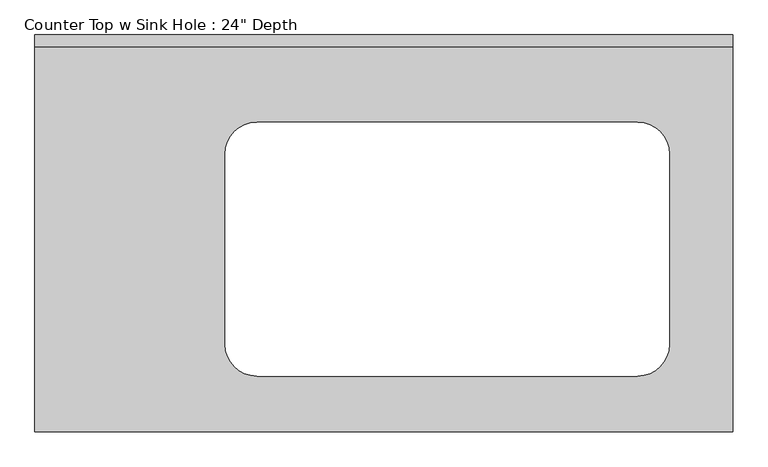
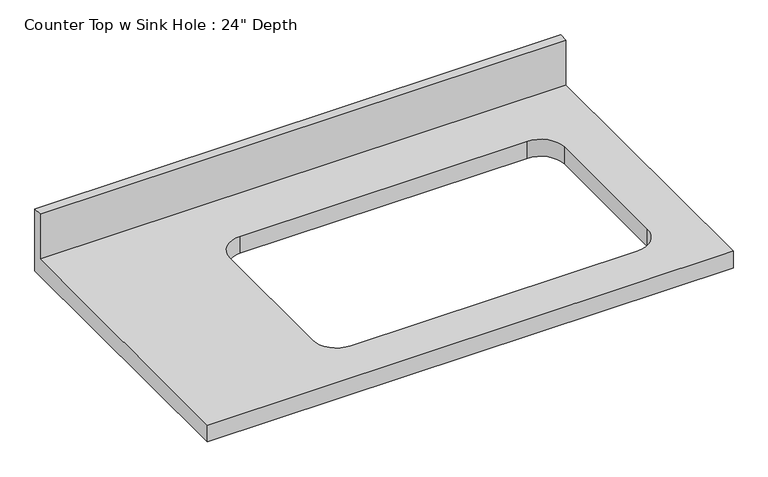
"""IFC4 building model written with IfcOpenShell, lengths in millimetres: furniture geometry."""

from ifc_helpers import new_model, si_unit, frame, origin, place, context, project, spatial, polyline, circle_curve, source, transform, mapped, element, save
from ifc_brep_helpers import plane_surface, revolved_surface, advanced_brep


def furniture_a6d59748(model_context):
    return source(origin(), model_context, "Body", "AdvancedBrep", [
        advanced_brep(
        [(-1200.4622951, -635.0, 914.4), (-82.8622951, -635.0, 914.4), (-82.8622951, -19.05, 914.4), (-1200.4622951, -19.05, 914.4), (-844.8622951, -139.7, 914.4), (-235.2622951, -139.7, 914.4), (-184.4622951, -190.5, 914.4), (-184.4622951, -495.3, 914.4), (-235.2622951, -546.1, 914.4), (-844.8622951, -546.1, 914.4), (-895.6622951, -495.3, 914.4), (-895.6622951, -190.5, 914.4), (-82.8622951, 0.0, 876.3), (-82.8622951, -635.0, 876.3), (-1200.4622951, -635.0, 876.3), (-1200.4622951, 0.0, 876.3), (-235.2622951, -139.7, 876.3), (-844.8622951, -139.7, 876.3), (-895.6622951, -190.5, 876.3), (-895.6622951, -495.3, 876.3), (-844.8622951, -546.1, 876.3), (-235.2622951, -546.1, 876.3), (-184.4622951, -495.3, 876.3), (-184.4622951, -190.5, 876.3), (-1200.4622951, 0.0, 1016.0), (-82.8622951, 0.0, 1016.0), (-1200.4622951, -19.05, 1016.0), (-82.8622951, -19.05, 1016.0)],
        [
            (0, 1),
            (1, 2),
            (2, 3),
            (3, 0),
            (4, 5),
            (5, 6, circle_curve(frame((-235.2622951, -190.5, 914.4), z_axis=(0.0, 0.0, -1.0), x_axis=(1.0, 0.0, 0.0)), 50.8)),
            (6, 7),
            (7, 8, circle_curve(frame((-235.2622951, -495.3, 914.4), z_axis=(0.0, 0.0, -1.0), x_axis=(1.0, 0.0, 0.0)), 50.8)),
            (8, 9),
            (9, 10, circle_curve(frame((-844.8622951, -495.3, 914.4), z_axis=(0.0, 0.0, -1.0), x_axis=(1.0, 0.0, 0.0)), 50.8)),
            (10, 11),
            (11, 4, circle_curve(frame((-844.8622951, -190.5, 914.4), z_axis=(0.0, 0.0, -1.0), x_axis=(1.0, 0.0, 0.0)), 50.8)),
            (12, 13),
            (13, 14),
            (14, 15),
            (15, 12),
            (16, 17),
            (17, 18, circle_curve(frame((-844.8622951, -190.5, 876.3), z_axis=(0.0, 0.0, 1.0), x_axis=(1.0, 0.0, 0.0)), 50.8)),
            (18, 19),
            (19, 20, circle_curve(frame((-844.8622951, -495.3, 876.3), z_axis=(0.0, 0.0, 1.0), x_axis=(1.0, 0.0, 0.0)), 50.8)),
            (20, 21),
            (21, 22, circle_curve(frame((-235.2622951, -495.3, 876.3), z_axis=(0.0, 0.0, 1.0), x_axis=(1.0, 0.0, 0.0)), 50.8)),
            (22, 23),
            (23, 16, circle_curve(frame((-235.2622951, -190.5, 876.3), z_axis=(0.0, 0.0, 1.0), x_axis=(1.0, 0.0, 0.0)), 50.8)),
            (15, 24),
            (24, 25),
            (25, 12),
            (14, 0),
            (3, 26),
            (26, 24),
            (13, 1),
            (25, 27),
            (27, 2),
            (26, 27),
            (4, 17),
            (16, 5),
            (11, 18),
            (10, 19),
            (9, 20),
            (8, 21),
            (7, 22),
            (6, 23),
        ],
        [
            plane_surface(frame((-1200.4622951, 0.0, 914.4), z_axis=(0.0, 0.0, 1.0), x_axis=(-1.0, 0.0, 0.0))),
            plane_surface(frame((-1200.4622951, 0.0, 876.3), z_axis=(0.0, 0.0, -1.0), x_axis=(1.0, 0.0, 0.0))),
            plane_surface(frame((-82.8622951, 0.0, 914.4), z_axis=(0.0, 1.0, 0.0), x_axis=(0.0, 0.0, -1.0))),
            plane_surface(frame((-1200.4622951, 0.0, 914.4), z_axis=(-1.0, 0.0, 0.0), x_axis=(0.0, 0.0, -1.0))),
            plane_surface(frame((-1200.4622951, -635.0, 914.4), z_axis=(0.0, -1.0, 0.0), x_axis=(0.0, 0.0, -1.0))),
            plane_surface(frame((-82.8622951, -635.0, 914.4), z_axis=(1.0, 0.0, 0.0), x_axis=(0.0, 0.0, -1.0))),
            plane_surface(frame((-1200.4622951, 0.0, 1016.0), z_axis=(0.0, 0.0, 1.0), x_axis=(0.0, -1.0, 0.0))),
            plane_surface(frame((-1200.4622951, -19.05, 1016.0), z_axis=(0.0, -1.0, 0.0), x_axis=(0.0, 0.0, -1.0))),
            plane_surface(frame((-235.2622951, -139.7, 914.4), z_axis=(0.0, -1.0, 0.0), x_axis=(0.0, 0.0, -1.0))),
            revolved_surface(polyline([(-794.0622951, -190.5, 914.4), (-794.0622951, -190.5, 876.3)]), (-844.8622951, -190.5, 876.3), (0.0, 0.0, 1.0)),
            plane_surface(frame((-895.6622951, -190.5, 914.4), z_axis=(1.0, 0.0, 0.0), x_axis=(0.0, 0.0, -1.0))),
            revolved_surface(polyline([(-794.0622951, -495.3, 914.4), (-794.0622951, -495.3, 876.3)]), (-844.8622951, -495.3, 876.3), (0.0, 0.0, 1.0)),
            plane_surface(frame((-844.8622951, -546.1, 914.4), z_axis=(0.0, 1.0, 0.0), x_axis=(0.0, 0.0, -1.0))),
            revolved_surface(polyline([(-184.4622951, -495.3, 914.4), (-184.4622951, -495.3, 876.3)]), (-235.2622951, -495.3, 876.3), (0.0, 0.0, 1.0)),
            plane_surface(frame((-184.4622951, -495.3, 914.4), z_axis=(-1.0, 0.0, 0.0), x_axis=(0.0, 0.0, -1.0))),
            revolved_surface(polyline([(-184.4622951, -190.5, 914.4), (-184.4622951, -190.5, 876.3)]), (-235.2622951, -190.5, 876.3), (0.0, 0.0, 1.0)),
        ],
        [
            (0, [[1, 2, 3, 4], [5, 6, 7, 8, 9, 10, 11, 12]]),
            (1, [[13, 14, 15, 16], [17, 18, 19, 20, 21, 22, 23, 24]]),
            (2, [[-16, 25, 26, 27]]),
            (3, [[-15, 28, -4, 29, 30, -25]]),
            (4, [[-1, -28, -14, 31]]),
            (5, [[-13, -27, 32, 33, -2, -31]]),
            (6, [[-30, 34, -32, -26]]),
            (7, [[-34, -29, -3, -33]]),
            (8, [[35, -17, 36, -5]]),
            (9, [[-35, -12, 37, -18]]),
            (10, [[-37, -11, 38, -19]]),
            (11, [[-38, -10, 39, -20]]),
            (12, [[-39, -9, 40, -21]]),
            (13, [[-40, -8, 41, -22]]),
            (14, [[-41, -7, 42, -23]]),
            (15, [[-36, -24, -42, -6]]),
        ],
    ),
    ])


if __name__ == "__main__":
    model = new_model("IFC4")
    model_context = context("Model", 3, world=origin())
    ifc_project = project(units=[si_unit("LENGTHUNIT", "METRE", prefix="MILLI")], contexts=[model_context])
    site = spatial("IfcSite", under=ifc_project)
    building = spatial("IfcBuilding", under=site)
    placement = place(None, origin())
    furniture_shape = furniture_a6d59748(model_context)
    element("IfcFurniture", 1, ObjectType="Counter Top w Sink Hole : 24\" Depth", at=placement, inside=building, context=model_context, shape_type="MappedRepresentation", body=[
        mapped(furniture_shape, transform((0.0, 0.0, 0.0), x_axis=(1.0, 0.0, 0.0), y_axis=(0.0, 1.0, 0.0), z_axis=(0.0, 0.0, 1.0))),
    ])
    save(model, "model.ifc")

# Revit data of these elements
# Type "Counter Top w Sink Hole : 24\" Depth"
#   Assembly Code = "C1030400"
#   Counter Thickness = 0' - 1 1/2"
#   Depth = 2' - 1"
#   Height = 3' - 0"
#   Length [instance default] = 8' - 0"
#   Sink Location [instance default] = 2' - 0"
#   Sink Location To Wall [instance default] = 0' - 6"
#   Sink Opening Depth [instance default] = 1' - 3"
#   Sink Opening Width [instance default] = 2' - 3"
#   Counter Top Material = none
#   Default Elevation = 0
# Element 1 (IfcFurniture, "Counter Top w Sink Hole : 24\" Depth")
#   Length = 3' - 8"
#   Sink Location = 2' - 2"
#   Materials on its faces: "Counter Top"
# Materials
#   "Counter Top": class "Wood", colour RGB 226 177 128, transparency 0
